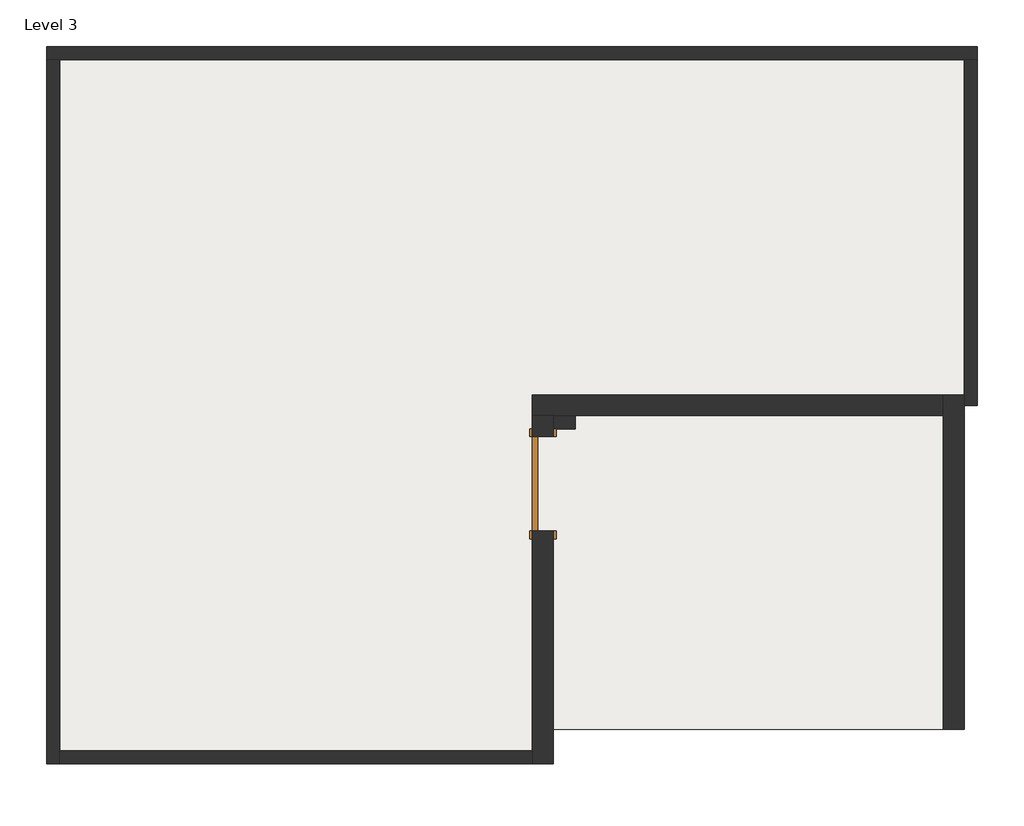
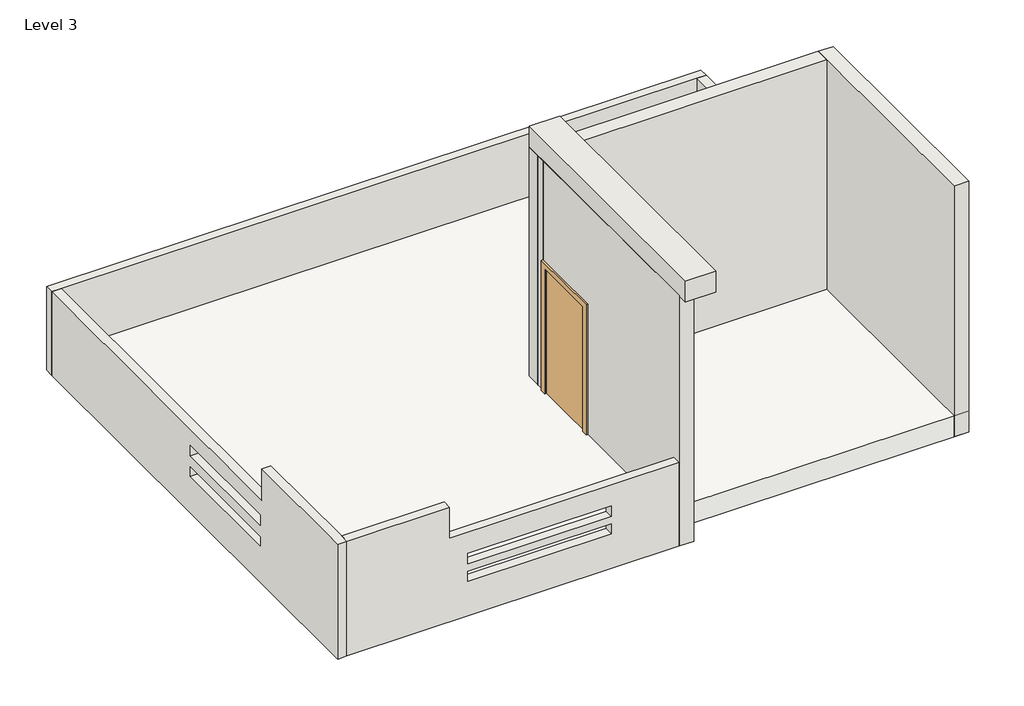
# One storey: 8 walls, 1 door, 1 roof.
"""IFC4 building model written with IfcOpenShell, lengths in millimetres."""

from ifc_helpers import new_model, si_unit, frame, origin, place, context, project, spatial, polyline, outline, extrude, faceted_brep, transform, mapped, element, save
from components import door_54dd4da4, walls_2_walls_2_c4a6eebc

model = new_model("IFC4")

# Units and contexts
model_context = context("Model", 3, world=origin())
ifc_project = project(units=[si_unit("LENGTHUNIT", "METRE", prefix="MILLI")], contexts=[model_context])

# Site, building, storey
site = spatial("IfcSite", under=ifc_project)
building = spatial("IfcBuilding", under=site)
storey = spatial("IfcBuildingStorey", under=building, Name="Level 3", Elevation=7315.2)

# Door
placement = place(None, origin())
door_shape = door_54dd4da4(model_context)
element("IfcDoor", 1, ObjectType="Single-Flush : 36\" x 84\"", at=placement, inside=storey, context=model_context, shape_type="MappedRepresentation", body=[
    mapped(door_shape, transform((-6878.4236868, 8277.1756066, 7315.2), x_axis=(0.0, 1.0, 0.0), y_axis=(-1.0, 0.0, 0.0), z_axis=(0.0, 0.0, 1.0))),
])

# Roof
element("IfcRoof", 2, ObjectType="Generic - 12\"", at=placement, inside=storey, context=model_context, shape_type="SweptSolid", body=[
    extrude(outline(polyline([(-11593.749546, 12388.334124), (-2789.0236868, 12388.334124), (-2789.0236868, 5893.2170892), (-6776.8236868, 5893.2170892), (-6776.8236868, 5686.3756066), (-11593.749546, 5686.3756066), (-11593.749546, 9187.934124), (-11593.749546, 12388.334124)])), frame((0.0, 0.0, 7315.2), z_axis=(0.0, 0.0, 1.0), x_axis=(1.0, 0.0, 0.0)), (0.0, 0.0, 1.0), 304.8),
])

# Walls
element("IfcWall", 3, ObjectType="Generic - 5\"", at=placement, inside=storey, context=model_context, shape_type="Brep", body=[
    faceted_brep([(-11695.349546, 12395.6170892, 7315.2), (-11695.349546, 5559.3756066, 7315.2), (-11695.349546, 5559.3756066, 8534.4), (-11695.349546, 5559.3756066, 8991.6), (-11695.349546, 7375.4756066, 8991.6), (-11695.349546, 7375.4756066, 8534.4), (-11695.349546, 12395.6170892, 8534.4), (-11695.349546, 7413.6760007, 8293.5144908), (-11695.349546, 7413.6760007, 8141.1144908), (-11695.349546, 9090.0760007, 8141.1144908), (-11695.349546, 9090.0760007, 8293.5144908), (-11695.349546, 7413.6760007, 7977.8098448), (-11695.349546, 7413.6760007, 7844.0949743), (-11695.349546, 9090.0760007, 7844.0949743), (-11695.349546, 9090.0760007, 7977.8098448), (-11568.349546, 12395.6170892, 7315.2), (-11568.349546, 12395.6170892, 8534.4), (-11568.349546, 7375.4756066, 8534.4), (-11568.349546, 7375.4756066, 8991.6), (-11568.349546, 5686.3756066, 8991.6), (-11568.349546, 5559.3756066, 8991.6), (-11568.349546, 5559.3756066, 8534.4), (-11568.349546, 5559.3756066, 7315.2), (-11568.349546, 5686.3756066, 7315.2), (-11568.349546, 7413.6760007, 8293.5144908), (-11568.349546, 9090.0760007, 8293.5144908), (-11568.349546, 9090.0760007, 8141.1144908), (-11568.349546, 7413.6760007, 8141.1144908), (-11568.349546, 7413.6760007, 7977.8098448), (-11568.349546, 9090.0760007, 7977.8098448), (-11568.349546, 9090.0760007, 7844.0949743), (-11568.349546, 7413.6760007, 7844.0949743), (-11593.749546, 12395.6170892, 7315.2)], [[[0, 1, 2, 3, 4, 5, 6], [7, 8, 9, 10], [11, 12, 13, 14]], [[15, 16, 17, 18, 19, 20, 21, 22, 23], [24, 25, 26, 27], [28, 29, 30, 31]], [[0, 6, 16, 15, 32]], [[1, 0, 32, 15, 23, 22]], [[6, 5, 17, 16]], [[8, 7, 24, 27]], [[9, 8, 27, 26]], [[10, 9, 26, 25]], [[7, 10, 25, 24]], [[12, 11, 28, 31]], [[13, 12, 31, 30]], [[14, 13, 30, 29]], [[11, 14, 29, 28]], [[4, 3, 20, 19, 18]], [[5, 4, 18, 17]], [[3, 2, 1, 22, 21, 20]]]),
])
element("IfcWall", 4, ObjectType="Generic - 5\"", at=placement, inside=storey, context=model_context, shape_type="Brep", body=[
    faceted_brep([(-11568.349546, 5559.3756066, 7315.2), (-6980.0236868, 5559.3756066, 7315.2), (-6980.0236868, 5559.3756066, 8534.4), (-10152.299546, 5559.3756066, 8534.4), (-10152.299546, 5559.3756066, 8991.6), (-11568.349546, 5559.3756066, 8991.6), (-11568.349546, 5559.3756066, 8534.4), (-7917.099546, 5559.3756066, 8226.5227428), (-7917.099546, 5559.3756066, 8074.1227428), (-9898.299546, 5559.3756066, 8074.1227428), (-9898.299546, 5559.3756066, 8226.5227428), (-7917.099546, 5559.3756066, 7964.4050931), (-7917.099546, 5559.3756066, 7820.8178766), (-9898.299546, 5559.3756066, 7820.8178766), (-9898.299546, 5559.3756066, 7964.4050931), (-11568.349546, 5686.3756066, 7315.2), (-11568.349546, 5686.3756066, 8534.4), (-11568.349546, 5686.3756066, 8991.6), (-10152.299546, 5686.3756066, 8991.6), (-10152.299546, 5686.3756066, 8534.4), (-6980.0236868, 5686.3756066, 8534.4), (-6980.0236868, 5686.3756066, 7315.2), (-7917.099546, 5686.3756066, 8226.5227428), (-9898.299546, 5686.3756066, 8226.5227428), (-9898.299546, 5686.3756066, 8074.1227428), (-7917.099546, 5686.3756066, 8074.1227428), (-7917.099546, 5686.3756066, 7964.4050931), (-9898.299546, 5686.3756066, 7964.4050931), (-9898.299546, 5686.3756066, 7820.8178766), (-7917.099546, 5686.3756066, 7820.8178766)], [[[0, 1, 2, 3, 4, 5, 6], [7, 8, 9, 10], [11, 12, 13, 14]], [[15, 16, 17, 18, 19, 20, 21], [22, 23, 24, 25], [26, 27, 28, 29]], [[2, 1, 21, 20]], [[1, 0, 15, 21]], [[3, 2, 20, 19]], [[8, 7, 22, 25]], [[9, 8, 25, 24]], [[10, 9, 24, 23]], [[7, 10, 23, 22]], [[12, 11, 26, 29]], [[13, 12, 29, 28]], [[14, 13, 28, 27]], [[11, 14, 27, 26]], [[4, 3, 19, 18]], [[5, 4, 18, 17]], [[6, 5, 17, 16, 15, 0]]]),
])
element("IfcWall", 5, ObjectType="Generic - 5\"", at=placement, inside=storey, context=model_context, shape_type="Brep", body=[
    faceted_brep([(-11695.349546, 12395.6170892, 7315.2), (-11568.349546, 12395.6170892, 7315.2), (-2789.0236868, 12395.6170892, 7315.2), (-2662.0236868, 12395.6170892, 7315.2), (-2662.0236868, 12395.6170892, 8534.4), (-2789.0236868, 12395.6170892, 8534.4), (-11568.349546, 12395.6170892, 8534.4), (-11695.349546, 12395.6170892, 8534.4), (-11695.349546, 12522.6170892, 7315.2), (-11695.349546, 12522.6170892, 8534.4), (-2662.0236868, 12522.6170892, 8534.4), (-2662.0236868, 12522.6170892, 7315.2)], [[[0, 1, 2, 3, 4, 5, 6, 7]], [[8, 9, 10, 11]], [[3, 2, 1, 0, 8, 11]], [[7, 6, 5, 4, 10, 9]], [[4, 3, 11, 10]], [[0, 7, 9, 8]]]),
])
element("IfcWall", 6, ObjectType="Generic - 5\"", at=placement, inside=storey, context=model_context, shape_type="Brep", body=[
    faceted_brep([(-2789.0236868, 12395.6170892, 7315.2), (-2789.0236868, 9039.1756066, 7315.2), (-2789.0236868, 9039.1756066, 8534.4), (-2789.0236868, 12395.6170892, 8534.4), (-2662.0236868, 12395.6170892, 7315.2), (-2662.0236868, 12395.6170892, 8534.4), (-2662.0236868, 9039.1756066, 8534.4), (-2662.0236868, 9039.1756066, 7315.2), (-2779.949546, 12395.6170892, 7315.2)], [[[0, 1, 2, 3]], [[4, 5, 6, 7]], [[1, 0, 8, 4, 7]], [[2, 1, 7, 6]], [[3, 2, 6, 5]], [[0, 3, 5, 4, 8]]]),
])
element("IfcWall", 7, ObjectType="Generic - 8\"", at=placement, inside=storey, context=model_context, shape_type="Brep", body=[
    faceted_brep([(-2789.0236868, 5893.2170892, 7315.2), (-2789.0236868, 9140.7756066, 7315.2), (-2789.0236868, 9140.7756066, 10972.8), (-2789.0236868, 5893.2170892, 10972.8), (-2992.2236868, 5893.2170892, 7315.2), (-2992.2236868, 5893.2170892, 10972.8), (-2992.2236868, 8937.5756066, 10972.8), (-2992.2236868, 9140.7756066, 10972.8), (-2992.2236868, 9140.7756066, 7315.2), (-2992.2236868, 8937.5756066, 7315.2), (-2983.149546, 5893.2170892, 7315.2)], [[[0, 1, 2, 3]], [[4, 5, 6, 7, 8, 9]], [[1, 0, 10, 4, 9, 8]], [[0, 3, 5, 4, 10]], [[3, 2, 7, 6, 5]], [[2, 1, 8, 7]]]),
])
element("IfcWall", 8, ObjectType="Generic - 8\"", at=placement, inside=storey, context=model_context, shape_type="Brep", body=[
    faceted_brep([(-2992.2236868, 9140.7756066, 7315.2), (-6980.0236868, 9140.7756066, 7315.2), (-6980.0236868, 9140.7756066, 10972.8), (-2992.2236868, 9140.7756066, 10972.8), (-2992.2236868, 8937.5756066, 7315.2), (-2992.2236868, 8937.5756066, 10972.8), (-6776.8236868, 8937.5756066, 10972.8), (-6980.0236868, 8937.5756066, 10972.8), (-6980.0236868, 8937.5756066, 7315.2), (-6776.8236868, 8937.5756066, 7315.2)], [[[0, 1, 2, 3]], [[4, 5, 6, 7, 8, 9]], [[1, 0, 4, 9, 8]], [[2, 1, 8, 7]], [[3, 2, 7, 6, 5]], [[0, 3, 5, 4]]]),
])
element("IfcWall", 9, ObjectType="Generic - 8\"", at=placement, inside=storey, context=model_context, shape_type="Brep", body=[
    faceted_brep([(-6980.0236868, 8937.5756066, 7315.2), (-6980.0236868, 8734.3756066, 7315.2), (-6980.0236868, 8734.3756066, 9448.8), (-6980.0236868, 7819.9756066, 9448.8), (-6980.0236868, 7819.9756066, 7315.2), (-6980.0236868, 5686.3756066, 7315.2), (-6980.0236868, 5559.3756066, 7315.2), (-6980.0236868, 5559.3756066, 8534.4), (-6980.0236868, 5559.3756066, 10972.8), (-6980.0236868, 8937.5756066, 10972.8), (-6776.8236868, 8734.3756066, 9448.8), (-6776.8236868, 8734.3756066, 7315.2), (-6776.8236868, 8937.5756066, 7315.2), (-6776.8236868, 8937.5756066, 10972.8), (-6776.8236868, 5559.3756066, 10972.8), (-6776.8236868, 5559.3756066, 7315.2), (-6776.8236868, 7819.9756066, 7315.2), (-6776.8236868, 7819.9756066, 9448.8)], [[[0, 1, 2, 3, 4, 5, 6, 7, 8, 9]], [[10, 11, 12, 13, 14, 15, 16, 17]], [[16, 15, 6, 5, 4]], [[12, 11, 1, 0]], [[0, 9, 13, 12]], [[9, 8, 14, 13]], [[2, 1, 11, 10]], [[3, 2, 10, 17]], [[4, 3, 17, 16]], [[8, 7, 6, 15, 14]]]),
])
walls_2_walls_2_shape = walls_2_walls_2_c4a6eebc(model_context)
element("IfcWall", 10, ObjectType="Walls 2 : Walls 2", at=placement, inside=storey, context=model_context, shape_type="MappedRepresentation", body=[
    mapped(walls_2_walls_2_shape, transform((0.0, 0.0, 0.0), x_axis=(1.0, 0.0, 0.0), y_axis=(0.0, 1.0, 0.0), z_axis=(0.0, 0.0, 1.0))),
])

save(model, "model.ifc")

# Revit data of these elements
# Type "Single-Flush : 36\" x 84\""
#   Type Mark = "1"
#   Construction Type Id = "MDOOR"
#   Assembly Code = "C1020"
#   Analytic Construction = "Metal"
#   Thickness = 0' - 2"
#   Heat Transfer Coefficient (U) = 0.651978 BTU/(h·ft²·°F)
#   Height = 7' - 0"
#   Trim Projection Ext = 0' - 1"
#   Trim Projection Int = 0' - 1"
#   Trim Width = 0' - 3"
#   Width = 3' - 0"
#   Define Thermal Properties by = 1
#   Door Material = Door - Panel
#   Frame Material = Door - Frame
#   Visual Light Transmittance = 0
#   Solar Heat Gain Coefficient = 0
#   Function = (empty or 0)
#   Wall Closure = (empty or 0)
# Type "Generic - 12\""
#   Assembly Code = "B1020"
#   Layers, outside or top first: 1' - 0" no material (function 1)
# Type "Generic - 5\""
#   Assembly Code = "B2010"
#   Layers, outside or top first: 0' - 5" no material (function 1)
# Type "Generic - 8\""
#   Assembly Code = "B2010"
#   Layers, outside or top first: 0' - 8" no material (function 1)
# Element 1 (IfcDoor, "Single-Flush : 36\" x 84\"")
#   Phase Created = New Construction
#   Materials on its faces: "Door - Frame", "Door - Panel"
# Element 2 (IfcRoof, "Generic - 12\"")
#   built-in parameter 1001705 = 25 (stored number, unit not read)
#   built-in parameter 1001710 = 33615
#   Phase Created = New Construction
#   Materials on its faces: "Default Roof"
# Elements 3, 4, 5, 6 (IfcWall, "Generic - 5\"")
#   Top Offset = -8' - 0"
#   Base Offset = 0' - 0"
#   wall height = 4' - 0"
#   Phase Created = New Construction
#   Base Constraint = Level 3
#   Top Constraint = Level 4
#   Materials on its faces: "Default Wall"
# Elements 7, 8, 9 (IfcWall, "Generic - 8\"")
#   Top Offset = 0' - 0"
#   Base Offset = 0' - 0"
#   Unconnected Height = 12' - 0"
#   wall height = 12' - 0"
#   Phase Created = New Construction
#   Base Constraint = Level 3
#   Materials on its faces: "Default Wall"
# Element 10 (IfcWall, "Walls 2 : Walls 2")
#   Phase Created = New Construction
#   Materials on its faces: "Default Wall"
# Materials
#   "Door - Panel": class "Wood", colour RGB 210 159 95, transparency 0
#   "Door - Frame": colour RGB 118 70 51, transparency 0
#   "Default Roof": colour RGB 88 101 114, transparency 0
#   "Default Wall": colour RGB 128 128 128, transparency 0
